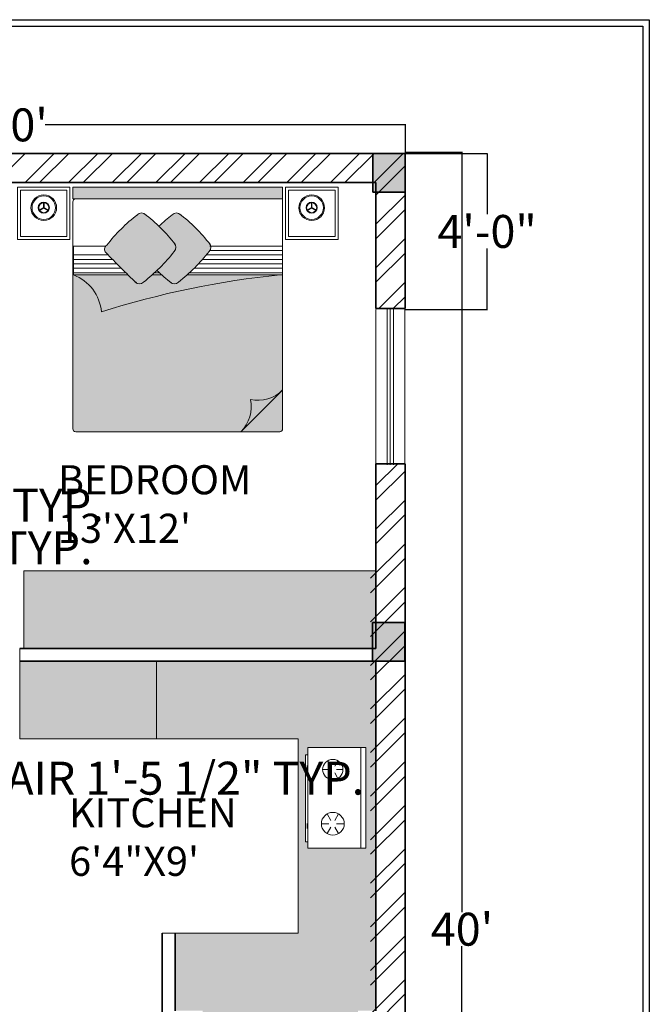
# Model space of a CAD drawing. Units: inches. Extents: x 1812 to 2791, y 2306 to 2959.
# Tile 8 of 8: x 2575 to 2770, y 2655 to 2959. Entities that reach past the tile are written whole.
import ezdxf

# ---------------------------------------------------------------- set-up
doc = ezdxf.new("R2010")
doc.units = ezdxf.units.IN
doc.layers.get('Defpoints').update_dxf_attribs({"lineweight": 50})
for name, color, linetype, lineweight in [('00 FURNITURE', 15, 'Continuous', 15), ('A-ANNO-DIMS', 2, 'Continuous', 18), ('A-ANNO-TTLB', 7, 'Continuous', 25), ('A-AREA-IDEN', 7, 'Continuous', 18), ('A-COLS', 7, 'Continuous', 35), ('A-EQPM', 8, 'Continuous', 18), ('A-FLOR-CASE', 8, 'Continuous', 18), ('A-WALL-PATT', 8, 'Continuous', 13), ('WALL', 7, 'Continuous', 35), ('WINDOWS', 160, 'Continuous', 18)]:
    doc.layers.add(name, color=color, linetype=linetype, lineweight=lineweight)
doc.layers.add('A-FURN-PATT', color=241, linetype='Continuous', lineweight=9, true_color=0xf7abae)
doc.layers.add('FURN3D', color=229, linetype='Continuous', lineweight=5, true_color=0x4a3f41)
doc.styles.get("Standard").update_dxf_attribs({"font": 'arial.ttf'})
doc.dimstyles.get("Standard").update_dxf_attribs({"dimtxt": 10.18, "dimasz": 0.18, "dimexe": 0.18, "dimexo": 0.0625, "dimgap": 0.09, "dimtad": 0, "dimtih": 1, "dimtoh": 1, "dimdec": 0, "dimzin": 0, "dimdsep": 46, "dimlunit": 3, "dimtxsty": 'Standard', "dimcen": 0.09, "dimadec": 0, "dimazin": 0, "dimtfac": 1, "dimtdec": 0, "dimtofl": 0, "dimtmove": 0, "dimatfit": 3, "dimfxl": 1, "dimtolj": 1, "dimtzin": 0, "dimarcsym": 0})

# ---------------------------------------------------------------- blocks, each defined once
blk = doc.blocks.new('RGWTG')
at = {"layer": '00 FURNITURE'}
for p, q in [((578.23, 3473.51), (577.36, 3475.01)), ((578.23, 3473.58), (577.36, 3472.08)), ((578.36, 3473.58), (577.49, 3475.09)), ((578.36, 3473.51), (577.49, 3472)), ((578.29, 3473.62), (580.03, 3473.62)), ((578.29, 3473.47), (580.03, 3473.47)), ((521.93, 3464.58), (509.03, 3451.68)), ((509.03, 3422.63), (509.03, 3463.68)), ((509.93, 3464.58), (566.4, 3464.58)), ((557.53, 3463.84), (557.53, 3464.49)), ((557.53, 3464.49), (566.4, 3464.49)), ((558.2, 3464.49), (558.2, 3435.82)), ((559.57, 3464.49), (559.57, 3437.25)), ((560.94, 3464.49), (560.94, 3438.58)), ((562.3, 3464.49), (562.3, 3439.83)), ((563.67, 3464.49), (563.67, 3440.99)), ((565.04, 3464.49), (565.04, 3442.08)), ((566.4, 3464.58), (580.98, 3464.58)), ((566.4, 3464.49), (566.4, 3442.08)), ((566.4, 3464.49), (566.4, 3463.84)), ((580.98, 3464.58), (580.98, 3416.72)), ((558.2, 3426.48), (558.2, 3425.04)), ((509.03, 3400.68), (509.03, 3422.63)), ((558.2, 3416.13), (558.2, 3399.95)), ((559.57, 3414.75), (559.57, 3399.95)), ((580.98, 3416.72), (580.98, 3400.68)), ((560.94, 3413.39), (560.94, 3399.95)), ((562.3, 3412.04), (562.3, 3399.95)), ((563.67, 3410.72), (563.67, 3399.95)), ((580.08, 3399.78), (509.93, 3399.78)), ((557.53, 3399.95), (557.53, 3400.6)), ((566.4, 3399.95), (557.53, 3399.95)), ((566.4, 3400.6), (566.4, 3399.95)), ((578.23, 3390.78), (577.36, 3392.29)), ((578.23, 3390.86), (577.36, 3389.36)), ((578.36, 3390.86), (577.49, 3392.36)), ((578.36, 3390.78), (577.49, 3389.28)), ((578.29, 3390.9), (580.03, 3390.9)), ((578.29, 3390.74), (580.03, 3390.74))]:
    blk.add_line(p, q, dxfattribs=at)
for points in [[(568.43, 3465.48), (584.63, 3465.48), (584.63, 3481.68), (568.43, 3481.68)], [(569.33, 3466.38), (583.73, 3466.38), (583.73, 3480.78), (569.33, 3480.78)], [(580.98, 3399.78), (584.63, 3399.78), (584.63, 3464.58), (580.98, 3464.58)], [(568.43, 3398.88), (584.63, 3398.88), (584.63, 3382.68), (568.43, 3382.68)], [(569.33, 3397.98), (583.73, 3397.98), (583.73, 3383.58), (569.33, 3383.58)]]:
    blk.add_lwpolyline(points, close=True, dxfattribs=at)
for points in [[(566.52, 3464.49), (557.53, 3464.49), (557.53, 3435.08)], [(557.53, 3427.21), (557.53, 3424.3)], [(557.53, 3416.82), (557.53, 3399.95), (566.4, 3399.95), (566.4, 3409.94)]]:
    blk.add_lwpolyline(points, dxfattribs=at)
for centre, radius in [((578.29, 3473.54), 3.97), ((578.29, 3473.54), 3.63), ((578.29, 3473.54), 1.74), ((578.29, 3473.54), 1.56), ((578.29, 3390.82), 3.97), ((578.29, 3390.82), 3.63), ((578.29, 3390.82), 1.74), ((578.29, 3390.82), 1.56)]:
    blk.add_circle(centre, radius, dxfattribs=at)
for centre, radius, start, end in [((509.93, 3463.68), 0.9, 90, 180), ((529.65, 3456.88), 10.9, 135.0361, 191.9278), ((290.56, 3490.52), 268.3, 342.2214, 354.2925), ((516.73, 3443.97), 10.9, 78.0722, 134.9639), ((566.05, 3440.57), 1.82, 45, 135), ((533.58, 3399.31), 54.32, 37.931, 52.069), ((598.15, 3399.01), 54.32, 127.931, 142.069), ((574.84, 3431.77), 1.82, 315, 45), ((556.59, 3431.11), 1.82, 135, 225), ((597.87, 3463.6), 54.32, 217.931, 224.141), ((598.15, 3388.23), 54.32, 127.931, 142.069), ((566.05, 3429.78), 1.82, 45, 135), ((533.58, 3388.53), 54.32, 37.931, 52.069), ((533.28, 3463.88), 54.32, 316.32, 322.069), ((556.59, 3420.33), 1.82, 135, 225), ((574.84, 3420.99), 1.82, 315, 45), ((765.33, 3619.75), 290.45, 223.6069, 226.2326), ((533.28, 3453.1), 54.32, 307.931, 322.069), ((565.44, 3411.05), 1.47, 225.9674, 326.8337), ((545.02, 3395.29), 13.35, 20.4224, 85.5825), ((509.93, 3400.68), 0.9, 180, 270), ((580.08, 3400.68), 0.9, 270, 0)]:
    blk.add_arc(centre, radius, start, end, dxfattribs=at)
blk = doc.blocks.new('A$C21540130')
at = {"layer": 'FURN3D'}
for p, q in [((1.57, 0), (1.57, 31.11)), ((9.61, 25.31), (8.63, 27.01)), ((10.79, 25.31), (11.77, 27.01)), ((9.02, 24.29, -27.54), (7.06, 24.29, -27.54)), ((9.61, 23.27), (8.63, 21.57)), ((10.79, 23.27), (11.77, 21.57)), ((11.38, 24.29, -27.54), (13.34, 24.29, -27.54)), ((9.61, 8.56), (8.43, 10.6)), ((10.79, 8.56), (11.97, 10.6)), ((9.02, 7.54), (6.67, 7.54)), ((9.61, 6.52), (8.43, 4.48)), ((10.79, 6.52), (11.97, 4.48)), ((11.38, 7.54), (13.73, 7.54))]:
    blk.add_line(p, q, dxfattribs=at)
for points in [[(0, 0), (0, 31.11), (17.9, 31.11), (17.9, 0)], [(18.68, 1.96), (18.68, 28.83), (17.9, 28.83), (17.9, 1.96)]]:
    blk.add_lwpolyline(points, close=True, dxfattribs=at)
for centre, radius in [((10.2, 24.29), 3.14), ((10.2, 7.54), 3.53)]:
    blk.add_circle(centre, radius, dxfattribs=at)
for points in [[(17.9, 24.03), (18.29, 24.03), (17.9, 25.6), (18.29, 25.6)], [(17.9, 6.05), (18.29, 6.05), (17.9, 7.62), (18.29, 7.62)]]:
    blk.add_solid(points, dxfattribs=at)
blk = doc.blocks.new('*D24')
at = {"layer": 'A-ANNO-DIMS', "color": 0, "lineweight": -2, "transparency": 16777216}
for p, q in [((2454.17, 2917.9), (2454.17, 2926.6)), ((2454.35, 2926.42), (2565.41, 2926.42)), ((2694.11, 2926.42), (2583.04, 2926.42)), ((2694.29, 2917.9), (2694.29, 2926.6))]:
    blk.add_line(p, q, dxfattribs=at)
at = {"layer": 'A-ANNO-DIMS', "color": 0, "transparency": 16777216}
for points in [[(2454.35, 2926.45), (2454.35, 2926.39), (2454.17, 2926.42)], [(2694.11, 2926.45), (2694.11, 2926.39), (2694.29, 2926.42)]]:
    blk.add_solid(points, dxfattribs=at)
at = {"layer": 'Defpoints', "color": 0, "transparency": 16777216}
for p in [(2694.29, 2926.42), (2454.17, 2917.83), (2694.29, 2917.83)]:
    blk.add_point(p, dxfattribs=at)
at = {"layer": 'A-ANNO-DIMS', "color": 0, "transparency": 16777216, "insert": (2574.23, 2926.42), "char_height": 10.18, "attachment_point": 5}
blk.add_mtext("\\A1;20'", dxfattribs=at)
blk = doc.blocks.new('*D25')
at = {"layer": 'A-ANNO-DIMS', "color": 0, "lineweight": -2, "transparency": 16777216}
for p, q in [((2694.21, 2918.01), (2711.94, 2918.01)), ((2711.76, 2917.83), (2711.76, 2683.09)), ((2711.76, 2437.78), (2711.76, 2672.52)), ((2694.21, 2437.6), (2711.94, 2437.6))]:
    blk.add_line(p, q, dxfattribs=at)
at = {"layer": 'A-ANNO-DIMS', "color": 0, "transparency": 16777216}
for points in [[(2711.73, 2917.83), (2711.79, 2917.83), (2711.76, 2918.01)], [(2711.73, 2437.78), (2711.79, 2437.78), (2711.76, 2437.6)]]:
    blk.add_solid(points, dxfattribs=at)
at = {"layer": 'Defpoints', "color": 0, "transparency": 16777216}
for p in [(2694.14, 2918.01), (2694.14, 2437.6), (2711.76, 2437.6)]:
    blk.add_point(p, dxfattribs=at)
at = {"layer": 'A-ANNO-DIMS', "color": 0, "transparency": 16777216, "insert": (2711.76, 2677.81), "char_height": 10.18, "attachment_point": 5}
blk.add_mtext("\\A1;40'", dxfattribs=at)
blk = doc.blocks.new('COL')
at = {"transparency": 33554687}
h = blk.add_hatch(color=256, dxfattribs=at)
h.dxf.hatch_style = 1
h.paths.add_polyline_path([(2424.4, 2829.24), (2424.4, 2839.24), (2412.4, 2839.24), (2412.4, 2829.24)])
for p, q in [((2412.4, 2839.24), (2424.4, 2839.24)), ((2412.4, 2839.24), (2412.4, 2829.24)), ((2424.4, 2839.24), (2424.4, 2829.24)), ((2412.4, 2829.24), (2424.4, 2829.24))]:
    blk.add_line(p, q)
blk = doc.blocks.new('WINDOW-48x9')
for p, q in [((0, 48), (0, 0)), ((3.5, 0), (3.5, 48)), ((4.5, 0), (4.5, 48)), ((5.5, 0), (5.5, 48)), ((9, 0), (9, 48))]:
    blk.add_line(p, q)
blk = doc.blocks.new('SHEET-FRAME-RESIDENCE')
blk.add_lwpolyline([(0, 632.8), (378.76, 632.8), (378.76, 0), (0, 0)], close=True)
blk.add_lwpolyline([(2, 71.32), (2, 630.8), (376.76, 630.8), (376.76, 71.32)])
blk = doc.blocks.new('*D58')
at = {"layer": 'A-ANNO-DIMS', "color": 0, "lineweight": -2, "transparency": 16777216}
for p, q in [((2533.67, 2818.77), (2536.75, 2818.77)), ((2536.57, 2818.59), (2536.57, 2814.26)), ((2536.57, 2799.21), (2536.57, 2803.55)), ((2533.67, 2799.03), (2536.75, 2799.03))]:
    blk.add_line(p, q, dxfattribs=at)
at = {"layer": 'A-ANNO-DIMS', "color": 0, "transparency": 16777216}
for points in [[(2536.54, 2818.59), (2536.6, 2818.59), (2536.57, 2818.77)], [(2536.54, 2799.21), (2536.6, 2799.21), (2536.57, 2799.03)]]:
    blk.add_solid(points, dxfattribs=at)
at = {"layer": 'Defpoints', "color": 0, "transparency": 16777216}
for p in [(2533.6, 2818.77), (2533.6, 2799.03), (2536.57, 2799.03)]:
    blk.add_point(p, dxfattribs=at)
at = {"layer": 'A-ANNO-DIMS', "color": 0, "transparency": 16777216, "insert": (2536.57, 2808.9), "char_height": 10.18, "attachment_point": 5}
blk.add_mtext('\\A1;BASIN 1\'-7 1/2" TYP.', dxfattribs=at)
blk = doc.blocks.new('*D61')
at = {"layer": 'A-ANNO-DIMS', "color": 0, "lineweight": -2, "transparency": 16777216}
for p, q in [((2505.24, 2790.81), (2505.24, 2795.9)), ((2505.42, 2795.72), (2535.06, 2795.72)), ((2535.24, 2790.81), (2535.24, 2795.9)), ((2535.24, 2795.72), (2535.42, 2795.72))]:
    blk.add_line(p, q, dxfattribs=at)
at = {"layer": 'A-ANNO-DIMS', "color": 0, "transparency": 16777216}
for points in [[(2505.42, 2795.75), (2505.42, 2795.69), (2505.24, 2795.72)], [(2535.06, 2795.75), (2535.06, 2795.69), (2535.24, 2795.72)]]:
    blk.add_solid(points, dxfattribs=at)
at = {"layer": 'Defpoints', "color": 0, "transparency": 16777216}
for p in [(2535.24, 2795.72), (2505.24, 2790.75), (2535.24, 2790.75)]:
    blk.add_point(p, dxfattribs=at)
at = {"layer": 'A-ANNO-DIMS', "color": 0, "transparency": 16777216, "insert": (2566.62, 2795.72), "char_height": 10.18, "attachment_point": 5}
blk.add_mtext('\\A1;2\'-6" TYP.', dxfattribs=at)
blk = doc.blocks.new('*D64')
at = {"layer": 'A-ANNO-DIMS', "color": 0, "lineweight": -2, "transparency": 16777216}
for p, q in [((2499.74, 2721.9), (2499.74, 2724.67)), ((2499.92, 2724.49), (2517.21, 2724.49)), ((2517.39, 2721.9), (2517.39, 2724.67)), ((2517.39, 2724.49), (2517.57, 2724.49))]:
    blk.add_line(p, q, dxfattribs=at)
at = {"layer": 'A-ANNO-DIMS', "color": 0, "transparency": 16777216}
for points in [[(2499.92, 2724.52), (2499.92, 2724.46), (2499.74, 2724.49)], [(2517.21, 2724.52), (2517.21, 2724.46), (2517.39, 2724.49)]]:
    blk.add_solid(points, dxfattribs=at)
at = {"layer": 'Defpoints', "color": 0, "transparency": 16777216}
for p in [(2517.39, 2724.49), (2499.74, 2721.84), (2517.39, 2721.84)]:
    blk.add_point(p, dxfattribs=at)
at = {"layer": 'A-ANNO-DIMS', "color": 0, "transparency": 16777216, "insert": (2601.37, 2724.49), "char_height": 10.18, "attachment_point": 5}
blk.add_mtext('\\A1;END CHAIR 1\'-5 1/2" TYP.', dxfattribs=at)
blk = doc.blocks.new('*D79')
at = {"layer": 'A-ANNO-DIMS', "color": 0, "lineweight": -2, "transparency": 16777216}
for p, q in [((2694.25, 2917.61), (2719.68, 2917.61)), ((2719.5, 2917.43), (2719.5, 2898.78)), ((2719.5, 2869.55), (2719.5, 2888.21)), ((2694.19, 2869.37), (2719.68, 2869.37))]:
    blk.add_line(p, q, dxfattribs=at)
at = {"layer": 'A-ANNO-DIMS', "color": 0, "transparency": 16777216}
for points in [[(2719.47, 2917.43), (2719.53, 2917.43), (2719.5, 2917.61)], [(2719.47, 2869.55), (2719.53, 2869.55), (2719.5, 2869.37)]]:
    blk.add_solid(points, dxfattribs=at)
at = {"layer": 'Defpoints', "color": 0, "transparency": 16777216}
for p in [(2694.19, 2917.61), (2694.13, 2869.37), (2719.5, 2869.37)]:
    blk.add_point(p, dxfattribs=at)
at = {"layer": 'A-ANNO-DIMS', "color": 0, "transparency": 16777216, "insert": (2719.5, 2893.49), "char_height": 10.18, "attachment_point": 5}
blk.add_mtext('\\A1;4\'-0"', dxfattribs=at)

msp = doc.modelspace()

# ---------------------------------------------------------------- hatches: boundary and pattern name
at = {"layer": 'A-FURN-PATT', "transparency": 33554534}
h = msp.add_hatch(color=256, dxfattribs=at)
h.dxf.hatch_style = 1
h.paths.add_polyline_path([(2685.19, 2760.61), (2617.42, 2760.61), (2617.42, 2736.61), (2661.19, 2736.61), (2661.19, 2676.61), (2623.19, 2676.61), (2623.19, 2652.61), (2631.67, 2652.61), (2631.67, 2651.78), (2679.67, 2651.78), (2679.67, 2652.61), (2685.19, 2652.61)])
h.paths.add_polyline_path([(2664.17, 2733.97), (2682.07, 2733.97), (2682.07, 2702.86), (2664.17, 2702.86), (2664.17, 2704.82), (2663.38, 2704.82), (2663.38, 2731.7), (2664.17, 2731.7)], flags=16)
h.paths.add_polyline_path([(2675.01, 2727.15, -1), (2668.73, 2727.15, -1)], flags=0)
h.paths.add_polyline_path([(2675.4, 2710.4, -1), (2668.34, 2710.4, -1)], flags=0)
h.paths.add_polyline_path([(2685.16, 2788.57), (2576.48, 2788.57), (2576.48, 2764.61), (2685.16, 2764.61)])
h.paths.add_polyline_path([(2617.42, 2760.61), (2575.19, 2760.61), (2575.19, 2736.61), (2617.42, 2736.61)])
h.paths.add_polyline_path([(2499.24, 2557.09), (2472.96, 2557.09), (2472.96, 2530.81), (2499.24, 2530.81)])
h.paths.add_polyline_path([(2499.24, 2580.68, 0.414214), (2497.05, 2582.87), (2472.96, 2582.87), (2472.96, 2557.09), (2499.24, 2557.09)])
h.paths.add_polyline_path([(2529.89, 2601.46), (2503.61, 2601.46), (2503.61, 2577.37, 0.414214), (2505.8, 2575.18), (2527.7, 2575.18, 0.414214), (2529.89, 2577.37)])
h.paths.add_polyline_path([(2499.24, 2530.81), (2472.96, 2530.81), (2472.96, 2505.02), (2497.05, 2505.02, 0.414214), (2499.24, 2507.21)])
h.paths.add_polyline_path([(2531.22, 2514.08, 0.414214), (2529.03, 2516.27), (2507.13, 2516.27, 0.414214), (2504.94, 2514.08), (2504.94, 2489.99), (2531.22, 2489.99)])
h.paths.add_polyline_path([(2613.92, 2898.81, 0.308459), (2611.87, 2898.95, 0.065472), (2601.84, 2888.94), (2601.74, 2888.94, 0.386143), (2601.79, 2886.97, 0.011497), (2611.24, 2877.54, 0.265248), (2613.05, 2877.56, 0.066056), (2623.16, 2887.66, 0.308904), (2623.02, 2889.71, 0.059418)])
h.paths.add_polyline_path([(2624.7, 2898.81, 0.308459), (2622.65, 2898.95, 0.027227), (2618.16, 2895.1, -0.033416), (2623.02, 2889.72, -0.379362), (2622.88, 2887.3, -0.036525), (2617.56, 2881.42, 0.027343), (2622.04, 2877.53, 0.262295), (2623.83, 2877.56, 0.066056), (2633.94, 2887.66, 0.308904), (2633.8, 2889.71, 0.059418)])
h.paths.add_polyline_path([(2656.38, 2844.47), (2643.48, 2831.57), (2655.48, 2831.57, 0.414214), (2656.38, 2832.47)], flags=17)
h.paths.add_polyline_path([(2656.38, 2880.07), (2655.64, 2880.07, 0.052719), (2600.4, 2868.59, 0.295777), (2591.58, 2880.13), (2591.58, 2832.47, 0.414214), (2592.48, 2831.57), (2614.43, 2831.57), (2643.48, 2831.57, 0.253465), (2646.43, 2841.52, 0.253465), (2656.38, 2844.47)])
h.paths.add_polyline_path([(2655.64, 2880.07), (2626.88, 2880.07, -0.016036), (2624.2, 2877.84, -0.429576), (2621.56, 2877.91, -0.015371), (2619.01, 2880.07), (2616.1, 2880.07, -0.016036), (2613.42, 2877.84, -0.334836), (2611.24, 2877.54, -0.003141), (2608.62, 2880.07), (2591.75, 2880.07, -0.292232), (2600.4, 2868.59, -0.052719)], flags=17)
h.paths.add_polyline_path([(2656.39, 2844.48, -0.2538), (2646.43, 2841.52, -0.253465), (2643.48, 2831.57)])
h.paths.add_polyline_path([(2656.38, 2907.17), (2591.58, 2907.17), (2591.58, 2903.52), (2656.38, 2903.52)])
at = {"layer": 'A-WALL-PATT'}
h = msp.add_hatch(dxfattribs=at)
h.set_pattern_fill('ANSI32', color=256)
h.set_pattern_definition([(45, (563.806, 20.011), (-6.735192, 6.735192), []), (45, (568.296, 20.011), (-6.735192, 6.735192), [])])
h.paths.add_polyline_path([(2694.19, 2437.61), (2683.5, 2437.61), (2683.5, 2788.57), (2685.19, 2788.57), (2685.19, 2821.64), (2685.13, 2869.37), (2685.13, 2821.64), (2694.19, 2821.64)])
h.paths.add_polyline_path([(2587.19, 2446.61), (2463.19, 2446.61), (2463.19, 2473.61), (2515.61, 2473.61), (2515.61, 2477.61), (2463.19, 2477.61), (2463.19, 2610.61), (2523.74, 2610.61), (2523.74, 2614.61), (2463.19, 2614.61), (2463.19, 2654.54), (2454.19, 2654.54), (2454.19, 2437.61), (2587.19, 2437.61)])
h.paths.add_polyline_path([(2683.5, 2446.61), (2676.19, 2446.61), (2676.19, 2437.61), (2683.5, 2437.61)])
h.paths.add_polyline_path([(2463.19, 2760.61), (2505.19, 2760.61), (2505.19, 2764.61), (2463.19, 2764.61), (2463.19, 2792.95), (2454.19, 2792.95), (2454.19, 2702.54), (2463.02, 2702.54), (2463.02, 2702.65)])
h.paths.add_polyline_path([(2539.19, 2858.61), (2463.19, 2858.61), (2463.19, 2876.35), (2454.19, 2876.35), (2454.19, 2816.96), (2463.19, 2816.96), (2463.19, 2854.61), (2535.19, 2854.61), (2535.19, 2760.61), (2539.19, 2760.61)])
h.paths.add_polyline_path([(2683.5, 2917.61), (2454.19, 2917.61), (2454.19, 2900.37), (2463.19, 2900.37), (2463.19, 2908.61), (2683.5, 2908.61)])
h.paths.add_polyline_path([(2694.19, 2917.61), (2683.5, 2917.61), (2683.5, 2908.61), (2685.19, 2908.61), (2685.19, 2869.64), (2694.19, 2869.64)])

# ---------------------------------------------------------------- linework, layer by layer
at = {"layer": 'A-FLOR-CASE'}
for p, q in [((2685.16, 2788.57), (2576.48, 2788.57)), ((2576.48, 2764.61), (2576.48, 2788.57)), ((2685.16, 2764.57), (2685.16, 2788.57)), ((2575.19, 2736.61), (2575.19, 2764.61)), ((2617.42, 2736.61), (2617.42, 2760.61)), ((2575.19, 2736.61), (2661.19, 2736.61)), ((2661.19, 2736.61), (2661.19, 2676.61)), ((2619.19, 2676.61), (2661.19, 2676.61))]:
    msp.add_line(p, q, dxfattribs=at)
at = {"layer": 'WALL'}
for p, q in [((2454.19, 2917.61), (2694.19, 2917.61)), ((2694.19, 2917.61), (2694.19, 2869.64)), ((2463.19, 2908.61), (2685.19, 2908.61)), ((2685.19, 2908.61), (2685.19, 2869.64)), ((2685.19, 2869.64), (2694.19, 2869.64)), ((2685.19, 2821.64), (2685.19, 2764.61)), ((2685.19, 2821.64), (2685.19, 2764.61)), ((2685.19, 2821.64), (2694.19, 2821.64)), ((2694.19, 2821.64), (2694.19, 2437.61)), ((2575.19, 2764.61), (2685.19, 2764.61)), ((2575.19, 2760.61), (2619.19, 2760.61)), ((2575.19, 2760.61), (2685.19, 2760.61)), ((2685.19, 2760.61), (2685.19, 2652.61)), ((2619.19, 2648.61), (2619.19, 2676.61)), ((2623.19, 2652.61), (2623.19, 2676.61))]:
    msp.add_line(p, q, dxfattribs=at)

# ---------------------------------------------------------------- block references
at = {"layer": '00 FURNITURE', "xscale": -1, "rotation": 270}
msp.add_blockref('RGWTG', (-808.2, 2322.54), dxfattribs=at)
at = {"layer": 'A-ANNO-TTLB'}
msp.add_blockref('SHEET-FRAME-RESIDENCE', (2390.83, 2326.13), dxfattribs=at)
at = {"layer": 'A-COLS', "rotation": 270}
for p in [(-144.99, 5329.98), (-145.15, 5185.05)]:
    msp.add_blockref('COL', p, dxfattribs=at)
at = {"layer": 'A-EQPM', "xscale": -1}
msp.add_blockref('A$C21540130', (2682.07, 2702.86), dxfattribs=at)
at = {"layer": 'WINDOWS'}
msp.add_blockref('WINDOW-48x9', (2685.13, 2821.37), dxfattribs=at)

# ---------------------------------------------------------------- texts
at = {"layer": 'A-AREA-IDEN', "char_height": 9, "attachment_point": 1}
for s, insert in [("BEDROOM\\P13'X12'", (2586.97, 2821.23)), ('KITCHEN\\P6\'4"X9\'', (2590.44, 2718.3))]:
    msp.add_mtext_dynamic_manual_height_columns(s, width=96.4869, gutter_width=12.5, heights=[0], dxfattribs=dict(at, insert=insert))

# ---------------------------------------------------------------- dimensions: what is measured, and where the dimension line sits
at = {"layer": 'A-ANNO-DIMS'}
dim = msp.add_linear_dim(base=(2694.29, 2926.42), p1=(2454.17, 2917.83), p2=(2694.29, 2917.83), dimstyle='Standard', override={"dimclrd": 0, "dimclre": 0, "dimclrt": 0}, dxfattribs=at)
dim.commit()
dim.dimension.update_dxf_attribs({"geometry": '*D24', "text_midpoint": (2574.23, 2926.42)})
dim = msp.add_linear_dim(base=(2719.5, 2869.37), p1=(2694.19, 2917.61), p2=(2694.13, 2869.37), angle=90, dimstyle='Standard', override={"dimdec": 1, "dimlfac": 1, "dimrnd": 0, "dimzin": 1, "dimdsep": 46, "dimlunit": 4, "dimfrac": 2}, dxfattribs=at)
dim.commit()
dim.dimension.update_dxf_attribs({"geometry": '*D79', "text_midpoint": (2719.5, 2893.49)})
dim = msp.add_linear_dim(base=(2711.76, 2437.6), p1=(2694.14, 2918.01), p2=(2694.14, 2437.6), angle=90, dimstyle='Standard', override={"dimclrd": 0, "dimclre": 0, "dimclrt": 0}, dxfattribs=at)
dim.commit()
dim.dimension.update_dxf_attribs({"geometry": '*D25', "text_midpoint": (2711.76, 2677.81), "dimtype": 160})
dim = msp.add_linear_dim(base=(2536.57, 2799.03), p1=(2533.6, 2818.77), p2=(2533.6, 2799.03), angle=270, text='BASIN <> TYP.', dimstyle='Standard', override={"dimdec": 1, "dimlfac": 1, "dimrnd": 0, "dimzin": 1, "dimdsep": 46, "dimlunit": 4, "dimfrac": 2}, dxfattribs=at)
dim.commit()
dim.dimension.update_dxf_attribs({"geometry": '*D58', "text_midpoint": (2536.57, 2808.9)})
for base, p1, p2, text, picture, middle in [((2535.24, 2795.72), (2505.24, 2790.75), (2535.24, 2790.75), '<> TYP.', '*D61', (2566.62, 2795.72)), ((2517.3921, 2724.4878), (2499.7369, 2721.8395), (2517.3921, 2721.8395), 'END CHAIR <> TYP.', '*D64', (2601.3693, 2724.4878))]:
    dim = msp.add_linear_dim(base=base, p1=p1, p2=p2, text=text, dimstyle='Standard', override={"dimdec": 1, "dimlfac": 1, "dimrnd": 0, "dimzin": 1, "dimdsep": 46, "dimlunit": 4, "dimfrac": 2}, dxfattribs=at)
    dim.commit()
    dim.dimension.update_dxf_attribs({"geometry": picture, "text_midpoint": middle})

doc.saveas('drawing.dxf')
